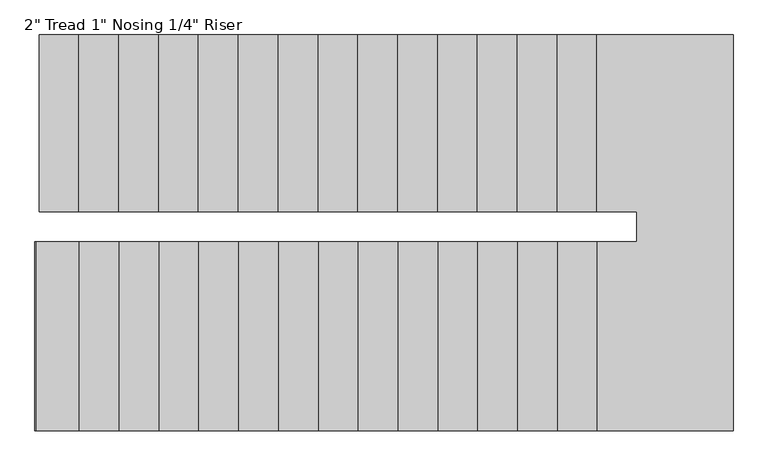
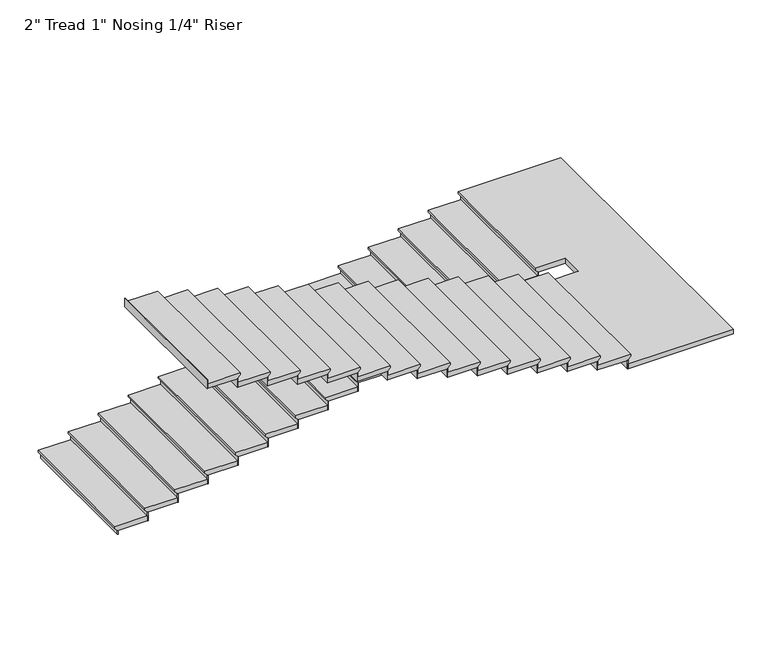
"""IFC4 building model written with IfcOpenShell, lengths in millimetres: stair flight geometry."""

from ifc_helpers import new_model, si_unit, origin, place, context, project, spatial, faceted_brep, source, transform, mapped, element, save


def stair_flight_b8102c9e(model_context):
    return source(origin(), model_context, "Body", "Brep", [
        faceted_brep([(-5254.0891351, 11154.2082924, 6168.39), (-5254.0891351, 11154.2082924, 6187.44), (-5254.0891351, 12506.0715905, 6187.44), (-5254.0891351, 12506.0715905, 6168.39), (-5228.6891351, 11154.2082924, 6142.99), (-5228.6891351, 12506.0715905, 6142.99), (-4923.8891351, 11154.2082924, 6187.44), (-4923.8891351, 12506.0715905, 6187.44), (-5228.6891351, 12506.0715905, 6136.64), (-4923.8891351, 12506.0715905, 6136.64), (-4923.8891351, 11154.2082924, 6136.64), (-5228.6891351, 11154.2082924, 6136.64)], [[[0, 1, 2, 3]], [[4, 0, 3, 5]], [[2, 1, 6, 7]], [[8, 9, 10, 11]], [[2, 7, 9, 8, 5, 3]], [[8, 11, 4, 5]], [[6, 1, 0, 4, 11, 10]], [[7, 6, 10, 9]]]),
        faceted_brep([(-5228.6891351, 11154.2082924, 6136.64), (-5228.6891351, 11154.2082924, 6096.0), (-5222.3391351, 11154.2082924, 6096.0), (-5222.3391351, 11154.2082924, 6136.64), (-5228.6891351, 12506.0715905, 6136.64), (-5222.3391351, 12506.0715905, 6136.64), (-5222.3391351, 12506.0715905, 6096.0), (-5228.6891351, 12506.0715905, 6096.0)], [[[0, 1, 2, 3]], [[4, 5, 6, 7]], [[1, 0, 4, 7]], [[2, 1, 7, 6]], [[3, 2, 6, 5]], [[0, 3, 5, 4]]]),
        faceted_brep([(-4923.8891351, 11154.2082924, 6228.08), (-4923.8891351, 11154.2082924, 6136.64), (-4917.5391351, 11154.2082924, 6136.64), (-4917.5391351, 11154.2082924, 6228.08), (-4923.8891351, 12506.0715905, 6228.08), (-4917.5391351, 12506.0715905, 6228.08), (-4917.5391351, 12506.0715905, 6136.64), (-4923.8891351, 12506.0715905, 6136.64)], [[[0, 1, 2, 3]], [[4, 5, 6, 7]], [[1, 0, 4, 7]], [[2, 1, 7, 6]], [[3, 2, 6, 5]], [[0, 3, 5, 4]]]),
        faceted_brep([(-4949.2891351, 12506.0715905, 6278.88), (-4949.2891351, 11154.2082924, 6278.88), (-4619.0891351, 11154.2082924, 6278.88), (-4619.0891351, 12506.0715905, 6278.88), (-4923.8891351, 12506.0715905, 6228.08), (-4619.0891351, 12506.0715905, 6228.08), (-4619.0891351, 11154.2082924, 6228.08), (-4923.8891351, 11154.2082924, 6228.08), (-4923.8891351, 12506.0715905, 6234.43), (-4949.2891351, 12506.0715905, 6259.83), (-4923.8891351, 11154.2082924, 6234.43), (-4949.2891351, 11154.2082924, 6259.83)], [[[0, 1, 2, 3]], [[4, 5, 6, 7]], [[0, 3, 5, 4, 8, 9]], [[4, 7, 10, 8]], [[2, 1, 11, 10, 7, 6]], [[3, 2, 6, 5]], [[11, 1, 0, 9]], [[10, 11, 9, 8]]]),
        faceted_brep([(-4619.0891351, 11154.2082924, 6319.52), (-4619.0891351, 11154.2082924, 6228.08), (-4612.7391351, 11154.2082924, 6228.08), (-4612.7391351, 11154.2082924, 6319.52), (-4619.0891351, 12506.0715905, 6319.52), (-4612.7391351, 12506.0715905, 6319.52), (-4612.7391351, 12506.0715905, 6228.08), (-4619.0891351, 12506.0715905, 6228.08)], [[[0, 1, 2, 3]], [[4, 5, 6, 7]], [[1, 0, 4, 7]], [[2, 1, 7, 6]], [[3, 2, 6, 5]], [[0, 3, 5, 4]]]),
        faceted_brep([(-4644.4891351, 12506.0715905, 6370.32), (-4644.4891351, 11154.2082924, 6370.32), (-4314.2891351, 11154.2082924, 6370.32), (-4314.2891351, 12506.0715905, 6370.32), (-4619.0891351, 12506.0715905, 6319.52), (-4314.2891351, 12506.0715905, 6319.52), (-4314.2891351, 11154.2082924, 6319.52), (-4619.0891351, 11154.2082924, 6319.52), (-4619.0891351, 12506.0715905, 6325.87), (-4644.4891351, 12506.0715905, 6351.27), (-4619.0891351, 11154.2082924, 6325.87), (-4644.4891351, 11154.2082924, 6351.27)], [[[0, 1, 2, 3]], [[4, 5, 6, 7]], [[0, 3, 5, 4, 8, 9]], [[4, 7, 10, 8]], [[2, 1, 11, 10, 7, 6]], [[3, 2, 6, 5]], [[11, 1, 0, 9]], [[10, 11, 9, 8]]]),
        faceted_brep([(-4314.2891351, 11154.2082924, 6410.96), (-4314.2891351, 11154.2082924, 6319.52), (-4307.9391351, 11154.2082924, 6319.52), (-4307.9391351, 11154.2082924, 6410.96), (-4314.2891351, 12506.0715905, 6410.96), (-4307.9391351, 12506.0715905, 6410.96), (-4307.9391351, 12506.0715905, 6319.52), (-4314.2891351, 12506.0715905, 6319.52)], [[[0, 1, 2, 3]], [[4, 5, 6, 7]], [[1, 0, 4, 7]], [[2, 1, 7, 6]], [[3, 2, 6, 5]], [[0, 3, 5, 4]]]),
        faceted_brep([(-4339.6891351, 12506.0715905, 6461.76), (-4339.6891351, 11154.2082924, 6461.76), (-4009.4891351, 11154.2082924, 6461.76), (-4009.4891351, 12506.0715905, 6461.76), (-4314.2891351, 12506.0715905, 6410.96), (-4009.4891351, 12506.0715905, 6410.96), (-4009.4891351, 11154.2082924, 6410.96), (-4314.2891351, 11154.2082924, 6410.96), (-4314.2891351, 12506.0715905, 6417.31), (-4339.6891351, 12506.0715905, 6442.71), (-4314.2891351, 11154.2082924, 6417.31), (-4339.6891351, 11154.2082924, 6442.71)], [[[0, 1, 2, 3]], [[4, 5, 6, 7]], [[0, 3, 5, 4, 8, 9]], [[4, 7, 10, 8]], [[2, 1, 11, 10, 7, 6]], [[3, 2, 6, 5]], [[11, 1, 0, 9]], [[10, 11, 9, 8]]]),
        faceted_brep([(-4009.4891351, 11154.2082924, 6502.4), (-4009.4891351, 11154.2082924, 6410.96), (-4003.1391351, 11154.2082924, 6410.96), (-4003.1391351, 11154.2082924, 6502.4), (-4009.4891351, 12506.0715905, 6502.4), (-4003.1391351, 12506.0715905, 6502.4), (-4003.1391351, 12506.0715905, 6410.96), (-4009.4891351, 12506.0715905, 6410.96)], [[[0, 1, 2, 3]], [[4, 5, 6, 7]], [[1, 0, 4, 7]], [[2, 1, 7, 6]], [[3, 2, 6, 5]], [[0, 3, 5, 4]]]),
        faceted_brep([(-4034.8891351, 12506.0715905, 6553.2), (-4034.8891351, 11154.2082924, 6553.2), (-3704.6891351, 11154.2082924, 6553.2), (-3704.6891351, 12506.0715905, 6553.2), (-4009.4891351, 12506.0715905, 6502.4), (-3704.6891351, 12506.0715905, 6502.4), (-3704.6891351, 11154.2082924, 6502.4), (-4009.4891351, 11154.2082924, 6502.4), (-4009.4891351, 12506.0715905, 6508.75), (-4034.8891351, 12506.0715905, 6534.15), (-4009.4891351, 11154.2082924, 6508.75), (-4034.8891351, 11154.2082924, 6534.15)], [[[0, 1, 2, 3]], [[4, 5, 6, 7]], [[0, 3, 5, 4, 8, 9]], [[4, 7, 10, 8]], [[2, 1, 11, 10, 7, 6]], [[3, 2, 6, 5]], [[11, 1, 0, 9]], [[10, 11, 9, 8]]]),
        faceted_brep([(-3704.6891351, 11154.2082924, 6593.84), (-3704.6891351, 11154.2082924, 6502.4), (-3698.3391351, 11154.2082924, 6502.4), (-3698.3391351, 11154.2082924, 6593.84), (-3704.6891351, 12506.0715905, 6593.84), (-3698.3391351, 12506.0715905, 6593.84), (-3698.3391351, 12506.0715905, 6502.4), (-3704.6891351, 12506.0715905, 6502.4)], [[[0, 1, 2, 3]], [[4, 5, 6, 7]], [[1, 0, 4, 7]], [[2, 1, 7, 6]], [[3, 2, 6, 5]], [[0, 3, 5, 4]]]),
        faceted_brep([(-3730.0891351, 12506.0715905, 6644.64), (-3730.0891351, 11154.2082924, 6644.64), (-3399.8891351, 11154.2082924, 6644.64), (-3399.8891351, 12506.0715905, 6644.64), (-3704.6891351, 12506.0715905, 6593.84), (-3399.8891351, 12506.0715905, 6593.84), (-3399.8891351, 11154.2082924, 6593.84), (-3704.6891351, 11154.2082924, 6593.84), (-3704.6891351, 12506.0715905, 6600.19), (-3730.0891351, 12506.0715905, 6625.59), (-3704.6891351, 11154.2082924, 6600.19), (-3730.0891351, 11154.2082924, 6625.59)], [[[0, 1, 2, 3]], [[4, 5, 6, 7]], [[0, 3, 5, 4, 8, 9]], [[4, 7, 10, 8]], [[2, 1, 11, 10, 7, 6]], [[3, 2, 6, 5]], [[11, 1, 0, 9]], [[10, 11, 9, 8]]]),
        faceted_brep([(-3399.8891351, 11154.2082924, 6685.28), (-3399.8891351, 11154.2082924, 6593.84), (-3393.5391351, 11154.2082924, 6593.84), (-3393.5391351, 11154.2082924, 6685.28), (-3399.8891351, 12506.0715905, 6685.28), (-3393.5391351, 12506.0715905, 6685.28), (-3393.5391351, 12506.0715905, 6593.84), (-3399.8891351, 12506.0715905, 6593.84)], [[[0, 1, 2, 3]], [[4, 5, 6, 7]], [[1, 0, 4, 7]], [[2, 1, 7, 6]], [[3, 2, 6, 5]], [[0, 3, 5, 4]]]),
        faceted_brep([(-3425.2891351, 12506.0715905, 6736.08), (-3425.2891351, 11154.2082924, 6736.08), (-3095.0891351, 11154.2082924, 6736.08), (-3095.0891351, 12506.0715905, 6736.08), (-3399.8891351, 12506.0715905, 6685.28), (-3095.0891351, 12506.0715905, 6685.28), (-3095.0891351, 11154.2082924, 6685.28), (-3399.8891351, 11154.2082924, 6685.28), (-3399.8891351, 12506.0715905, 6691.63), (-3425.2891351, 12506.0715905, 6717.03), (-3399.8891351, 11154.2082924, 6691.63), (-3425.2891351, 11154.2082924, 6717.03)], [[[0, 1, 2, 3]], [[4, 5, 6, 7]], [[0, 3, 5, 4, 8, 9]], [[4, 7, 10, 8]], [[2, 1, 11, 10, 7, 6]], [[3, 2, 6, 5]], [[11, 1, 0, 9]], [[10, 11, 9, 8]]]),
        faceted_brep([(-3095.0891351, 11154.2082924, 6776.72), (-3095.0891351, 11154.2082924, 6685.28), (-3088.7391351, 11154.2082924, 6685.28), (-3088.7391351, 11154.2082924, 6776.72), (-3095.0891351, 12506.0715905, 6776.72), (-3088.7391351, 12506.0715905, 6776.72), (-3088.7391351, 12506.0715905, 6685.28), (-3095.0891351, 12506.0715905, 6685.28)], [[[0, 1, 2, 3]], [[4, 5, 6, 7]], [[1, 0, 4, 7]], [[2, 1, 7, 6]], [[3, 2, 6, 5]], [[0, 3, 5, 4]]]),
        faceted_brep([(-3120.4891351, 12506.0715905, 6827.52), (-3120.4891351, 11154.2082924, 6827.52), (-2790.2891351, 11154.2082924, 6827.52), (-2790.2891351, 12506.0715905, 6827.52), (-3095.0891351, 12506.0715905, 6776.72), (-2790.2891351, 12506.0715905, 6776.72), (-2790.2891351, 11154.2082924, 6776.72), (-3095.0891351, 11154.2082924, 6776.72), (-3095.0891351, 12506.0715905, 6783.07), (-3120.4891351, 12506.0715905, 6808.47), (-3095.0891351, 11154.2082924, 6783.07), (-3120.4891351, 11154.2082924, 6808.47)], [[[0, 1, 2, 3]], [[4, 5, 6, 7]], [[0, 3, 5, 4, 8, 9]], [[4, 7, 10, 8]], [[2, 1, 11, 10, 7, 6]], [[3, 2, 6, 5]], [[11, 1, 0, 9]], [[10, 11, 9, 8]]]),
        faceted_brep([(-2790.2891351, 11154.2082924, 6868.16), (-2790.2891351, 11154.2082924, 6776.72), (-2783.9391351, 11154.2082924, 6776.72), (-2783.9391351, 11154.2082924, 6868.16), (-2790.2891351, 12506.0715905, 6868.16), (-2783.9391351, 12506.0715905, 6868.16), (-2783.9391351, 12506.0715905, 6776.72), (-2790.2891351, 12506.0715905, 6776.72)], [[[0, 1, 2, 3]], [[4, 5, 6, 7]], [[1, 0, 4, 7]], [[2, 1, 7, 6]], [[3, 2, 6, 5]], [[0, 3, 5, 4]]]),
        faceted_brep([(-2815.6891351, 12506.0715905, 6918.96), (-2815.6891351, 11154.2082924, 6918.96), (-2485.4891351, 11154.2082924, 6918.96), (-2485.4891351, 12506.0715905, 6918.96), (-2790.2891351, 12506.0715905, 6868.16), (-2485.4891351, 12506.0715905, 6868.16), (-2485.4891351, 11154.2082924, 6868.16), (-2790.2891351, 11154.2082924, 6868.16), (-2790.2891351, 12506.0715905, 6874.51), (-2815.6891351, 12506.0715905, 6899.91), (-2790.2891351, 11154.2082924, 6874.51), (-2815.6891351, 11154.2082924, 6899.91)], [[[0, 1, 2, 3]], [[4, 5, 6, 7]], [[0, 3, 5, 4, 8, 9]], [[4, 7, 10, 8]], [[2, 1, 11, 10, 7, 6]], [[3, 2, 6, 5]], [[11, 1, 0, 9]], [[10, 11, 9, 8]]]),
        faceted_brep([(-2485.4891351, 11154.2082924, 6959.6), (-2485.4891351, 11154.2082924, 6868.16), (-2479.1391351, 11154.2082924, 6868.16), (-2479.1391351, 11154.2082924, 6959.6), (-2485.4891351, 12506.0715905, 6959.6), (-2479.1391351, 12506.0715905, 6959.6), (-2479.1391351, 12506.0715905, 6868.16), (-2485.4891351, 12506.0715905, 6868.16)], [[[0, 1, 2, 3]], [[4, 5, 6, 7]], [[1, 0, 4, 7]], [[2, 1, 7, 6]], [[3, 2, 6, 5]], [[0, 3, 5, 4]]]),
        faceted_brep([(-2510.8891351, 12506.0715905, 7010.4), (-2510.8891351, 11154.2082924, 7010.4), (-2180.6891351, 11154.2082924, 7010.4), (-2180.6891351, 12506.0715905, 7010.4), (-2485.4891351, 12506.0715905, 6959.6), (-2180.6891351, 12506.0715905, 6959.6), (-2180.6891351, 11154.2082924, 6959.6), (-2485.4891351, 11154.2082924, 6959.6), (-2485.4891351, 12506.0715905, 6965.95), (-2510.8891351, 12506.0715905, 6991.35), (-2485.4891351, 11154.2082924, 6965.95), (-2510.8891351, 11154.2082924, 6991.35)], [[[0, 1, 2, 3]], [[4, 5, 6, 7]], [[0, 3, 5, 4, 8, 9]], [[4, 7, 10, 8]], [[2, 1, 11, 10, 7, 6]], [[3, 2, 6, 5]], [[11, 1, 0, 9]], [[10, 11, 9, 8]]]),
        faceted_brep([(-2180.6891351, 11154.2082924, 7051.04), (-2180.6891351, 11154.2082924, 6959.6), (-2174.3391351, 11154.2082924, 6959.6), (-2174.3391351, 11154.2082924, 7051.04), (-2180.6891351, 12506.0715905, 7051.04), (-2174.3391351, 12506.0715905, 7051.04), (-2174.3391351, 12506.0715905, 6959.6), (-2180.6891351, 12506.0715905, 6959.6)], [[[0, 1, 2, 3]], [[4, 5, 6, 7]], [[1, 0, 4, 7]], [[2, 1, 7, 6]], [[3, 2, 6, 5]], [[0, 3, 5, 4]]]),
        faceted_brep([(-2206.0891351, 12506.0715905, 7101.84), (-2206.0891351, 11154.2082924, 7101.84), (-1875.8891351, 11154.2082924, 7101.84), (-1875.8891351, 12506.0715905, 7101.84), (-2180.6891351, 12506.0715905, 7051.04), (-1875.8891351, 12506.0715905, 7051.04), (-1875.8891351, 11154.2082924, 7051.04), (-2180.6891351, 11154.2082924, 7051.04), (-2180.6891351, 12506.0715905, 7057.39), (-2206.0891351, 12506.0715905, 7082.79), (-2180.6891351, 11154.2082924, 7057.39), (-2206.0891351, 11154.2082924, 7082.79)], [[[0, 1, 2, 3]], [[4, 5, 6, 7]], [[0, 3, 5, 4, 8, 9]], [[4, 7, 10, 8]], [[2, 1, 11, 10, 7, 6]], [[3, 2, 6, 5]], [[11, 1, 0, 9]], [[10, 11, 9, 8]]]),
        faceted_brep([(-1875.8891351, 11154.2082924, 7142.48), (-1875.8891351, 11154.2082924, 7051.04), (-1869.5391351, 11154.2082924, 7051.04), (-1869.5391351, 11154.2082924, 7142.48), (-1875.8891351, 12506.0715905, 7142.48), (-1869.5391351, 12506.0715905, 7142.48), (-1869.5391351, 12506.0715905, 7051.04), (-1875.8891351, 12506.0715905, 7051.04)], [[[0, 1, 2, 3]], [[4, 5, 6, 7]], [[1, 0, 4, 7]], [[2, 1, 7, 6]], [[3, 2, 6, 5]], [[0, 3, 5, 4]]]),
        faceted_brep([(-1901.2891351, 12506.0715905, 7193.28), (-1901.2891351, 11154.2082924, 7193.28), (-1571.0891351, 11154.2082924, 7193.28), (-1571.0891351, 12506.0715905, 7193.28), (-1875.8891351, 12506.0715905, 7142.48), (-1571.0891351, 12506.0715905, 7142.48), (-1571.0891351, 11154.2082924, 7142.48), (-1875.8891351, 11154.2082924, 7142.48), (-1875.8891351, 12506.0715905, 7148.83), (-1901.2891351, 12506.0715905, 7174.23), (-1875.8891351, 11154.2082924, 7148.83), (-1901.2891351, 11154.2082924, 7174.23)], [[[0, 1, 2, 3]], [[4, 5, 6, 7]], [[0, 3, 5, 4, 8, 9]], [[4, 7, 10, 8]], [[2, 1, 11, 10, 7, 6]], [[3, 2, 6, 5]], [[11, 1, 0, 9]], [[10, 11, 9, 8]]]),
        faceted_brep([(-1571.0891351, 11154.2082924, 7233.92), (-1571.0891351, 11154.2082924, 7142.48), (-1564.7391351, 11154.2082924, 7142.48), (-1564.7391351, 11154.2082924, 7233.92), (-1571.0891351, 12506.0715905, 7233.92), (-1564.7391351, 12506.0715905, 7233.92), (-1564.7391351, 12506.0715905, 7142.48), (-1571.0891351, 12506.0715905, 7142.48)], [[[0, 1, 2, 3]], [[4, 5, 6, 7]], [[1, 0, 4, 7]], [[2, 1, 7, 6]], [[3, 2, 6, 5]], [[0, 3, 5, 4]]]),
        faceted_brep([(-1596.4891351, 12506.0715905, 7284.72), (-1596.4891351, 11154.2082924, 7284.72), (-1266.2891351, 11154.2082924, 7284.72), (-1266.2891351, 12506.0715905, 7284.72), (-1571.0891351, 12506.0715905, 7233.92), (-1266.2891351, 12506.0715905, 7233.92), (-1266.2891351, 11154.2082924, 7233.92), (-1571.0891351, 11154.2082924, 7233.92), (-1571.0891351, 12506.0715905, 7240.27), (-1596.4891351, 12506.0715905, 7265.67), (-1571.0891351, 11154.2082924, 7240.27), (-1596.4891351, 11154.2082924, 7265.67)], [[[0, 1, 2, 3]], [[4, 5, 6, 7]], [[0, 3, 5, 4, 8, 9]], [[4, 7, 10, 8]], [[2, 1, 11, 10, 7, 6]], [[3, 2, 6, 5]], [[11, 1, 0, 9]], [[10, 11, 9, 8]]]),
        faceted_brep([(-1266.2891351, 11154.2082924, 7325.36), (-1266.2891351, 11154.2082924, 7233.92), (-1259.9391351, 11154.2082924, 7233.92), (-1259.9391351, 11154.2082924, 7325.36), (-1266.2891351, 12506.0715905, 7325.36), (-1259.9391351, 12506.0715905, 7325.36), (-1259.9391351, 12506.0715905, 7233.92), (-1266.2891351, 12506.0715905, 7233.92)], [[[0, 1, 2, 3]], [[4, 5, 6, 7]], [[1, 0, 4, 7]], [[2, 1, 7, 6]], [[3, 2, 6, 5]], [[0, 3, 5, 4]]]),
        faceted_brep([(-1291.6891351, 12506.0715905, 7376.16), (-1291.6891351, 11154.2082924, 7376.16), (-961.4891351, 11154.2082924, 7376.16), (-961.4891351, 12506.0715905, 7376.16), (-1266.2891351, 12506.0715905, 7325.36), (-961.4891351, 12506.0715905, 7325.36), (-961.4891351, 11154.2082924, 7325.36), (-1266.2891351, 11154.2082924, 7325.36), (-1266.2891351, 12506.0715905, 7331.71), (-1291.6891351, 12506.0715905, 7357.11), (-1266.2891351, 11154.2082924, 7331.71), (-1291.6891351, 11154.2082924, 7357.11)], [[[0, 1, 2, 3]], [[4, 5, 6, 7]], [[0, 3, 5, 4, 8, 9]], [[4, 7, 10, 8]], [[2, 1, 11, 10, 7, 6]], [[3, 2, 6, 5]], [[11, 1, 0, 9]], [[10, 11, 9, 8]]]),
        faceted_brep([(-961.4891351, 11154.2082924, 7416.8), (-961.4891351, 11154.2082924, 7325.36), (-955.1391351, 11154.2082924, 7325.36), (-955.1391351, 11154.2082924, 7416.8), (-961.4891351, 12506.0715905, 7416.8), (-955.1391351, 12506.0715905, 7416.8), (-955.1391351, 12506.0715905, 7325.36), (-961.4891351, 12506.0715905, 7325.36)], [[[0, 1, 2, 3]], [[4, 5, 6, 7]], [[1, 0, 4, 7]], [[2, 1, 7, 6]], [[3, 2, 6, 5]], [[0, 3, 5, 4]]]),
        faceted_brep([(-1012.2891351, 9478.4949943, 7467.6), (54.5108649, 9478.4949943, 7467.6), (54.5108649, 12506.0715905, 7467.6), (-986.8891351, 12506.0715905, 7467.6), (-986.8891351, 11154.2082924, 7467.6), (-682.0891351, 11154.2082924, 7467.6), (-682.0891351, 10925.6082924, 7467.6), (-1012.2891351, 10925.6082924, 7467.6), (54.5108649, 9478.4949943, 7416.8), (-1012.2891351, 9478.4949943, 7416.8), (-1012.2891351, 10925.6082924, 7416.8), (-682.0891351, 10925.6082924, 7416.8), (-682.0891351, 11154.2082924, 7416.8), (-961.4891351, 11154.2082924, 7416.8), (-961.4891351, 12506.0715905, 7416.8), (54.5108649, 12506.0715905, 7416.8), (-961.4891351, 12506.0715905, 7423.15), (-986.8891351, 12506.0715905, 7448.55), (-961.4891351, 11154.2082924, 7423.15), (-986.8891351, 11154.2082924, 7448.55)], [[[0, 1, 2, 3, 4, 5, 6, 7]], [[8, 9, 10, 11, 12, 13, 14, 15]], [[1, 0, 9, 8]], [[2, 1, 8, 15]], [[3, 2, 15, 14, 16, 17]], [[14, 13, 18, 16]], [[5, 4, 19, 18, 13, 12]], [[6, 5, 12, 11]], [[7, 6, 11, 10]], [[0, 7, 10, 9]], [[19, 4, 3, 17]], [[18, 19, 17, 16]]]),
        faceted_brep([(-1012.2891351, 10925.6082924, 7508.24), (-1012.2891351, 10925.6082924, 7416.8), (-1018.6391351, 10925.6082924, 7416.8), (-1018.6391351, 10925.6082924, 7508.24), (-1012.2891351, 9478.4949943, 7508.24), (-1018.6391351, 9478.4949943, 7508.24), (-1018.6391351, 9478.4949943, 7416.8), (-1012.2891351, 9478.4949943, 7416.8)], [[[0, 1, 2, 3]], [[4, 5, 6, 7]], [[1, 0, 4, 7]], [[2, 1, 7, 6]], [[3, 2, 6, 5]], [[0, 3, 5, 4]]]),
        faceted_brep([(-986.8891351, 9478.4949943, 7559.04), (-986.8891351, 10925.6082924, 7559.04), (-1317.0891351, 10925.6082924, 7559.04), (-1317.0891351, 9478.4949943, 7559.04), (-1012.2891351, 9478.4949943, 7508.24), (-1317.0891351, 9478.4949943, 7508.24), (-1317.0891351, 10925.6082924, 7508.24), (-1012.2891351, 10925.6082924, 7508.24), (-1012.2891351, 9478.4949943, 7514.59), (-986.8891351, 9478.4949943, 7539.99), (-1012.2891351, 10925.6082924, 7514.59), (-986.8891351, 10925.6082924, 7539.99)], [[[0, 1, 2, 3]], [[4, 5, 6, 7]], [[0, 3, 5, 4, 8, 9]], [[4, 7, 10, 8]], [[2, 1, 11, 10, 7, 6]], [[3, 2, 6, 5]], [[11, 1, 0, 9]], [[10, 11, 9, 8]]]),
        faceted_brep([(-1317.0891351, 10925.6082924, 7599.68), (-1317.0891351, 10925.6082924, 7508.24), (-1323.4391351, 10925.6082924, 7508.24), (-1323.4391351, 10925.6082924, 7599.68), (-1317.0891351, 9478.4949943, 7599.68), (-1323.4391351, 9478.4949943, 7599.68), (-1323.4391351, 9478.4949943, 7508.24), (-1317.0891351, 9478.4949943, 7508.24)], [[[0, 1, 2, 3]], [[4, 5, 6, 7]], [[1, 0, 4, 7]], [[2, 1, 7, 6]], [[3, 2, 6, 5]], [[0, 3, 5, 4]]]),
        faceted_brep([(-1291.6891351, 9478.4949943, 7650.48), (-1291.6891351, 10925.6082924, 7650.48), (-1621.8891351, 10925.6082924, 7650.48), (-1621.8891351, 9478.4949943, 7650.48), (-1317.0891351, 9478.4949943, 7599.68), (-1621.8891351, 9478.4949943, 7599.68), (-1621.8891351, 10925.6082924, 7599.68), (-1317.0891351, 10925.6082924, 7599.68), (-1317.0891351, 9478.4949943, 7606.03), (-1291.6891351, 9478.4949943, 7631.43), (-1317.0891351, 10925.6082924, 7606.03), (-1291.6891351, 10925.6082924, 7631.43)], [[[0, 1, 2, 3]], [[4, 5, 6, 7]], [[0, 3, 5, 4, 8, 9]], [[4, 7, 10, 8]], [[2, 1, 11, 10, 7, 6]], [[3, 2, 6, 5]], [[11, 1, 0, 9]], [[10, 11, 9, 8]]]),
        faceted_brep([(-1621.8891351, 10925.6082924, 7691.12), (-1621.8891351, 10925.6082924, 7599.68), (-1628.2391351, 10925.6082924, 7599.68), (-1628.2391351, 10925.6082924, 7691.12), (-1621.8891351, 9478.4949943, 7691.12), (-1628.2391351, 9478.4949943, 7691.12), (-1628.2391351, 9478.4949943, 7599.68), (-1621.8891351, 9478.4949943, 7599.68)], [[[0, 1, 2, 3]], [[4, 5, 6, 7]], [[1, 0, 4, 7]], [[2, 1, 7, 6]], [[3, 2, 6, 5]], [[0, 3, 5, 4]]]),
        faceted_brep([(-1596.4891351, 9478.4949943, 7741.92), (-1596.4891351, 10925.6082924, 7741.92), (-1926.6891351, 10925.6082924, 7741.92), (-1926.6891351, 9478.4949943, 7741.92), (-1621.8891351, 9478.4949943, 7691.12), (-1926.6891351, 9478.4949943, 7691.12), (-1926.6891351, 10925.6082924, 7691.12), (-1621.8891351, 10925.6082924, 7691.12), (-1621.8891351, 9478.4949943, 7697.47), (-1596.4891351, 9478.4949943, 7722.87), (-1621.8891351, 10925.6082924, 7697.47), (-1596.4891351, 10925.6082924, 7722.87)], [[[0, 1, 2, 3]], [[4, 5, 6, 7]], [[0, 3, 5, 4, 8, 9]], [[4, 7, 10, 8]], [[2, 1, 11, 10, 7, 6]], [[3, 2, 6, 5]], [[11, 1, 0, 9]], [[10, 11, 9, 8]]]),
        faceted_brep([(-1926.6891351, 10925.6082924, 7782.56), (-1926.6891351, 10925.6082924, 7691.12), (-1933.0391351, 10925.6082924, 7691.12), (-1933.0391351, 10925.6082924, 7782.56), (-1926.6891351, 9478.4949943, 7782.56), (-1933.0391351, 9478.4949943, 7782.56), (-1933.0391351, 9478.4949943, 7691.12), (-1926.6891351, 9478.4949943, 7691.12)], [[[0, 1, 2, 3]], [[4, 5, 6, 7]], [[1, 0, 4, 7]], [[2, 1, 7, 6]], [[3, 2, 6, 5]], [[0, 3, 5, 4]]]),
        faceted_brep([(-1901.2891351, 9478.4949943, 7833.36), (-1901.2891351, 10925.6082924, 7833.36), (-2231.4891351, 10925.6082924, 7833.36), (-2231.4891351, 9478.4949943, 7833.36), (-1926.6891351, 9478.4949943, 7782.56), (-2231.4891351, 9478.4949943, 7782.56), (-2231.4891351, 10925.6082924, 7782.56), (-1926.6891351, 10925.6082924, 7782.56), (-1926.6891351, 9478.4949943, 7788.91), (-1901.2891351, 9478.4949943, 7814.31), (-1926.6891351, 10925.6082924, 7788.91), (-1901.2891351, 10925.6082924, 7814.31)], [[[0, 1, 2, 3]], [[4, 5, 6, 7]], [[0, 3, 5, 4, 8, 9]], [[4, 7, 10, 8]], [[2, 1, 11, 10, 7, 6]], [[3, 2, 6, 5]], [[11, 1, 0, 9]], [[10, 11, 9, 8]]]),
        faceted_brep([(-2231.4891351, 10925.6082924, 7874.0), (-2231.4891351, 10925.6082924, 7782.56), (-2237.8391351, 10925.6082924, 7782.56), (-2237.8391351, 10925.6082924, 7874.0), (-2231.4891351, 9478.4949943, 7874.0), (-2237.8391351, 9478.4949943, 7874.0), (-2237.8391351, 9478.4949943, 7782.56), (-2231.4891351, 9478.4949943, 7782.56)], [[[0, 1, 2, 3]], [[4, 5, 6, 7]], [[1, 0, 4, 7]], [[2, 1, 7, 6]], [[3, 2, 6, 5]], [[0, 3, 5, 4]]]),
        faceted_brep([(-2206.0891351, 9478.4949943, 7924.8), (-2206.0891351, 10925.6082924, 7924.8), (-2536.2891351, 10925.6082924, 7924.8), (-2536.2891351, 9478.4949943, 7924.8), (-2231.4891351, 9478.4949943, 7874.0), (-2536.2891351, 9478.4949943, 7874.0), (-2536.2891351, 10925.6082924, 7874.0), (-2231.4891351, 10925.6082924, 7874.0), (-2231.4891351, 9478.4949943, 7880.35), (-2206.0891351, 9478.4949943, 7905.75), (-2231.4891351, 10925.6082924, 7880.35), (-2206.0891351, 10925.6082924, 7905.75)], [[[0, 1, 2, 3]], [[4, 5, 6, 7]], [[0, 3, 5, 4, 8, 9]], [[4, 7, 10, 8]], [[2, 1, 11, 10, 7, 6]], [[3, 2, 6, 5]], [[11, 1, 0, 9]], [[10, 11, 9, 8]]]),
        faceted_brep([(-2536.2891351, 10925.6082924, 7965.44), (-2536.2891351, 10925.6082924, 7874.0), (-2542.6391351, 10925.6082924, 7874.0), (-2542.6391351, 10925.6082924, 7965.44), (-2536.2891351, 9478.4949943, 7965.44), (-2542.6391351, 9478.4949943, 7965.44), (-2542.6391351, 9478.4949943, 7874.0), (-2536.2891351, 9478.4949943, 7874.0)], [[[0, 1, 2, 3]], [[4, 5, 6, 7]], [[1, 0, 4, 7]], [[2, 1, 7, 6]], [[3, 2, 6, 5]], [[0, 3, 5, 4]]]),
        faceted_brep([(-2510.8891351, 9478.4949943, 8016.24), (-2510.8891351, 10925.6082924, 8016.24), (-2841.0891351, 10925.6082924, 8016.24), (-2841.0891351, 9478.4949943, 8016.24), (-2536.2891351, 9478.4949943, 7965.44), (-2841.0891351, 9478.4949943, 7965.44), (-2841.0891351, 10925.6082924, 7965.44), (-2536.2891351, 10925.6082924, 7965.44), (-2536.2891351, 9478.4949943, 7971.79), (-2510.8891351, 9478.4949943, 7997.19), (-2536.2891351, 10925.6082924, 7971.79), (-2510.8891351, 10925.6082924, 7997.19)], [[[0, 1, 2, 3]], [[4, 5, 6, 7]], [[0, 3, 5, 4, 8, 9]], [[4, 7, 10, 8]], [[2, 1, 11, 10, 7, 6]], [[3, 2, 6, 5]], [[11, 1, 0, 9]], [[10, 11, 9, 8]]]),
        faceted_brep([(-2841.0891351, 10925.6082924, 8056.88), (-2841.0891351, 10925.6082924, 7965.44), (-2847.4391351, 10925.6082924, 7965.44), (-2847.4391351, 10925.6082924, 8056.88), (-2841.0891351, 9478.4949943, 8056.88), (-2847.4391351, 9478.4949943, 8056.88), (-2847.4391351, 9478.4949943, 7965.44), (-2841.0891351, 9478.4949943, 7965.44)], [[[0, 1, 2, 3]], [[4, 5, 6, 7]], [[1, 0, 4, 7]], [[2, 1, 7, 6]], [[3, 2, 6, 5]], [[0, 3, 5, 4]]]),
        faceted_brep([(-2815.6891351, 9478.4949943, 8107.68), (-2815.6891351, 10925.6082924, 8107.68), (-3145.8891351, 10925.6082924, 8107.68), (-3145.8891351, 9478.4949943, 8107.68), (-2841.0891351, 9478.4949943, 8056.88), (-3145.8891351, 9478.4949943, 8056.88), (-3145.8891351, 10925.6082924, 8056.88), (-2841.0891351, 10925.6082924, 8056.88), (-2841.0891351, 9478.4949943, 8063.23), (-2815.6891351, 9478.4949943, 8088.63), (-2841.0891351, 10925.6082924, 8063.23), (-2815.6891351, 10925.6082924, 8088.63)], [[[0, 1, 2, 3]], [[4, 5, 6, 7]], [[0, 3, 5, 4, 8, 9]], [[4, 7, 10, 8]], [[2, 1, 11, 10, 7, 6]], [[3, 2, 6, 5]], [[11, 1, 0, 9]], [[10, 11, 9, 8]]]),
        faceted_brep([(-3145.8891351, 10925.6082924, 8148.32), (-3145.8891351, 10925.6082924, 8056.88), (-3152.2391351, 10925.6082924, 8056.88), (-3152.2391351, 10925.6082924, 8148.32), (-3145.8891351, 9478.4949943, 8148.32), (-3152.2391351, 9478.4949943, 8148.32), (-3152.2391351, 9478.4949943, 8056.88), (-3145.8891351, 9478.4949943, 8056.88)], [[[0, 1, 2, 3]], [[4, 5, 6, 7]], [[1, 0, 4, 7]], [[2, 1, 7, 6]], [[3, 2, 6, 5]], [[0, 3, 5, 4]]]),
        faceted_brep([(-3120.4891351, 9478.4949943, 8199.12), (-3120.4891351, 10925.6082924, 8199.12), (-3450.6891351, 10925.6082924, 8199.12), (-3450.6891351, 9478.4949943, 8199.12), (-3145.8891351, 9478.4949943, 8148.32), (-3450.6891351, 9478.4949943, 8148.32), (-3450.6891351, 10925.6082924, 8148.32), (-3145.8891351, 10925.6082924, 8148.32), (-3145.8891351, 9478.4949943, 8154.67), (-3120.4891351, 9478.4949943, 8180.07), (-3145.8891351, 10925.6082924, 8154.67), (-3120.4891351, 10925.6082924, 8180.07)], [[[0, 1, 2, 3]], [[4, 5, 6, 7]], [[0, 3, 5, 4, 8, 9]], [[4, 7, 10, 8]], [[2, 1, 11, 10, 7, 6]], [[3, 2, 6, 5]], [[11, 1, 0, 9]], [[10, 11, 9, 8]]]),
        faceted_brep([(-3450.6891351, 10925.6082924, 8239.76), (-3450.6891351, 10925.6082924, 8148.32), (-3457.0391351, 10925.6082924, 8148.32), (-3457.0391351, 10925.6082924, 8239.76), (-3450.6891351, 9478.4949943, 8239.76), (-3457.0391351, 9478.4949943, 8239.76), (-3457.0391351, 9478.4949943, 8148.32), (-3450.6891351, 9478.4949943, 8148.32)], [[[0, 1, 2, 3]], [[4, 5, 6, 7]], [[1, 0, 4, 7]], [[2, 1, 7, 6]], [[3, 2, 6, 5]], [[0, 3, 5, 4]]]),
        faceted_brep([(-3425.2891351, 9478.4949943, 8290.56), (-3425.2891351, 10925.6082924, 8290.56), (-3755.4891351, 10925.6082924, 8290.56), (-3755.4891351, 9478.4949943, 8290.56), (-3450.6891351, 9478.4949943, 8239.76), (-3755.4891351, 9478.4949943, 8239.76), (-3755.4891351, 10925.6082924, 8239.76), (-3450.6891351, 10925.6082924, 8239.76), (-3450.6891351, 9478.4949943, 8246.11), (-3425.2891351, 9478.4949943, 8271.51), (-3450.6891351, 10925.6082924, 8246.11), (-3425.2891351, 10925.6082924, 8271.51)], [[[0, 1, 2, 3]], [[4, 5, 6, 7]], [[0, 3, 5, 4, 8, 9]], [[4, 7, 10, 8]], [[2, 1, 11, 10, 7, 6]], [[3, 2, 6, 5]], [[11, 1, 0, 9]], [[10, 11, 9, 8]]]),
        faceted_brep([(-3755.4891351, 10925.6082924, 8331.2), (-3755.4891351, 10925.6082924, 8239.76), (-3761.8391351, 10925.6082924, 8239.76), (-3761.8391351, 10925.6082924, 8331.2), (-3755.4891351, 9478.4949943, 8331.2), (-3761.8391351, 9478.4949943, 8331.2), (-3761.8391351, 9478.4949943, 8239.76), (-3755.4891351, 9478.4949943, 8239.76)], [[[0, 1, 2, 3]], [[4, 5, 6, 7]], [[1, 0, 4, 7]], [[2, 1, 7, 6]], [[3, 2, 6, 5]], [[0, 3, 5, 4]]]),
        faceted_brep([(-3730.0891351, 9478.4949943, 8382.0), (-3730.0891351, 10925.6082924, 8382.0), (-4060.2891351, 10925.6082924, 8382.0), (-4060.2891351, 9478.4949943, 8382.0), (-3755.4891351, 9478.4949943, 8331.2), (-4060.2891351, 9478.4949943, 8331.2), (-4060.2891351, 10925.6082924, 8331.2), (-3755.4891351, 10925.6082924, 8331.2), (-3755.4891351, 9478.4949943, 8337.55), (-3730.0891351, 9478.4949943, 8362.95), (-3755.4891351, 10925.6082924, 8337.55), (-3730.0891351, 10925.6082924, 8362.95)], [[[0, 1, 2, 3]], [[4, 5, 6, 7]], [[0, 3, 5, 4, 8, 9]], [[4, 7, 10, 8]], [[2, 1, 11, 10, 7, 6]], [[3, 2, 6, 5]], [[11, 1, 0, 9]], [[10, 11, 9, 8]]]),
        faceted_brep([(-4060.2891351, 10925.6082924, 8422.64), (-4060.2891351, 10925.6082924, 8331.2), (-4066.6391351, 10925.6082924, 8331.2), (-4066.6391351, 10925.6082924, 8422.64), (-4060.2891351, 9478.4949943, 8422.64), (-4066.6391351, 9478.4949943, 8422.64), (-4066.6391351, 9478.4949943, 8331.2), (-4060.2891351, 9478.4949943, 8331.2)], [[[0, 1, 2, 3]], [[4, 5, 6, 7]], [[1, 0, 4, 7]], [[2, 1, 7, 6]], [[3, 2, 6, 5]], [[0, 3, 5, 4]]]),
        faceted_brep([(-4034.8891351, 9478.4949943, 8473.44), (-4034.8891351, 10925.6082924, 8473.44), (-4365.0891351, 10925.6082924, 8473.44), (-4365.0891351, 9478.4949943, 8473.44), (-4060.2891351, 9478.4949943, 8422.64), (-4365.0891351, 9478.4949943, 8422.64), (-4365.0891351, 10925.6082924, 8422.64), (-4060.2891351, 10925.6082924, 8422.64), (-4060.2891351, 9478.4949943, 8428.99), (-4034.8891351, 9478.4949943, 8454.39), (-4060.2891351, 10925.6082924, 8428.99), (-4034.8891351, 10925.6082924, 8454.39)], [[[0, 1, 2, 3]], [[4, 5, 6, 7]], [[0, 3, 5, 4, 8, 9]], [[4, 7, 10, 8]], [[2, 1, 11, 10, 7, 6]], [[3, 2, 6, 5]], [[11, 1, 0, 9]], [[10, 11, 9, 8]]]),
        faceted_brep([(-4365.0891351, 10925.6082924, 8514.08), (-4365.0891351, 10925.6082924, 8422.64), (-4371.4391351, 10925.6082924, 8422.64), (-4371.4391351, 10925.6082924, 8514.08), (-4365.0891351, 9478.4949943, 8514.08), (-4371.4391351, 9478.4949943, 8514.08), (-4371.4391351, 9478.4949943, 8422.64), (-4365.0891351, 9478.4949943, 8422.64)], [[[0, 1, 2, 3]], [[4, 5, 6, 7]], [[1, 0, 4, 7]], [[2, 1, 7, 6]], [[3, 2, 6, 5]], [[0, 3, 5, 4]]]),
        faceted_brep([(-4339.6891351, 9478.4949943, 8564.88), (-4339.6891351, 10925.6082924, 8564.88), (-4669.8891351, 10925.6082924, 8564.88), (-4669.8891351, 9478.4949943, 8564.88), (-4365.0891351, 9478.4949943, 8514.08), (-4669.8891351, 9478.4949943, 8514.08), (-4669.8891351, 10925.6082924, 8514.08), (-4365.0891351, 10925.6082924, 8514.08), (-4365.0891351, 9478.4949943, 8520.43), (-4339.6891351, 9478.4949943, 8545.83), (-4365.0891351, 10925.6082924, 8520.43), (-4339.6891351, 10925.6082924, 8545.83)], [[[0, 1, 2, 3]], [[4, 5, 6, 7]], [[0, 3, 5, 4, 8, 9]], [[4, 7, 10, 8]], [[2, 1, 11, 10, 7, 6]], [[3, 2, 6, 5]], [[11, 1, 0, 9]], [[10, 11, 9, 8]]]),
        faceted_brep([(-4669.8891351, 10925.6082924, 8605.52), (-4669.8891351, 10925.6082924, 8514.08), (-4676.2391351, 10925.6082924, 8514.08), (-4676.2391351, 10925.6082924, 8605.52), (-4669.8891351, 9478.4949943, 8605.52), (-4676.2391351, 9478.4949943, 8605.52), (-4676.2391351, 9478.4949943, 8514.08), (-4669.8891351, 9478.4949943, 8514.08)], [[[0, 1, 2, 3]], [[4, 5, 6, 7]], [[1, 0, 4, 7]], [[2, 1, 7, 6]], [[3, 2, 6, 5]], [[0, 3, 5, 4]]]),
        faceted_brep([(-4644.4891351, 9478.4949943, 8656.32), (-4644.4891351, 10925.6082924, 8656.32), (-4974.6891351, 10925.6082924, 8656.32), (-4974.6891351, 9478.4949943, 8656.32), (-4669.8891351, 9478.4949943, 8605.52), (-4974.6891351, 9478.4949943, 8605.52), (-4974.6891351, 10925.6082924, 8605.52), (-4669.8891351, 10925.6082924, 8605.52), (-4669.8891351, 9478.4949943, 8611.87), (-4644.4891351, 9478.4949943, 8637.27), (-4669.8891351, 10925.6082924, 8611.87), (-4644.4891351, 10925.6082924, 8637.27)], [[[0, 1, 2, 3]], [[4, 5, 6, 7]], [[0, 3, 5, 4, 8, 9]], [[4, 7, 10, 8]], [[2, 1, 11, 10, 7, 6]], [[3, 2, 6, 5]], [[11, 1, 0, 9]], [[10, 11, 9, 8]]]),
        faceted_brep([(-4974.6891351, 10925.6082924, 8696.96), (-4974.6891351, 10925.6082924, 8605.52), (-4981.0391351, 10925.6082924, 8605.52), (-4981.0391351, 10925.6082924, 8696.96), (-4974.6891351, 9478.4949943, 8696.96), (-4981.0391351, 9478.4949943, 8696.96), (-4981.0391351, 9478.4949943, 8605.52), (-4974.6891351, 9478.4949943, 8605.52)], [[[0, 1, 2, 3]], [[4, 5, 6, 7]], [[1, 0, 4, 7]], [[2, 1, 7, 6]], [[3, 2, 6, 5]], [[0, 3, 5, 4]]]),
        faceted_brep([(-5279.4891351, 10925.6082924, 8788.4), (-5279.4891351, 10925.6082924, 8696.96), (-5285.8391351, 10925.6082924, 8696.96), (-5285.8391351, 10925.6082924, 8788.4), (-5279.4891351, 9478.4949943, 8788.4), (-5285.8391351, 9478.4949943, 8788.4), (-5285.8391351, 9478.4949943, 8696.96), (-5279.4891351, 9478.4949943, 8696.96)], [[[0, 1, 2, 3]], [[4, 5, 6, 7]], [[1, 0, 4, 7]], [[2, 1, 7, 6]], [[3, 2, 6, 5]], [[0, 3, 5, 4]]]),
        faceted_brep([(-4949.2891351, 9478.4949943, 8747.76), (-4949.2891351, 10925.6082924, 8747.76), (-5279.4891351, 10925.6082924, 8747.76), (-5279.4891351, 9478.4949943, 8747.76), (-4974.6891351, 9478.4949943, 8696.96), (-5279.4891351, 9478.4949943, 8696.96), (-5279.4891351, 10925.6082924, 8696.96), (-4974.6891351, 10925.6082924, 8696.96), (-4974.6891351, 9478.4949943, 8703.31), (-4949.2891351, 9478.4949943, 8728.71), (-4974.6891351, 10925.6082924, 8703.31), (-4949.2891351, 10925.6082924, 8728.71)], [[[0, 1, 2, 3]], [[4, 5, 6, 7]], [[0, 3, 5, 4, 8, 9]], [[4, 7, 10, 8]], [[2, 1, 11, 10, 7, 6]], [[3, 2, 6, 5]], [[11, 1, 0, 9]], [[10, 11, 9, 8]]]),
    ])


if __name__ == "__main__":
    model = new_model("IFC4")
    model_context = context("Model", 3, world=origin())
    ifc_project = project(units=[si_unit("LENGTHUNIT", "METRE", prefix="MILLI")], contexts=[model_context])
    site = spatial("IfcSite", under=ifc_project)
    building = spatial("IfcBuilding", under=site)
    placement = place(None, origin())
    stair_flight_shape = stair_flight_b8102c9e(model_context)
    element("IfcStairFlight", 1, ObjectType="2\" Tread 1\" Nosing 1/4\" Riser", at=placement, inside=building, context=model_context, shape_type="MappedRepresentation", body=[
        mapped(stair_flight_shape, transform((0.0, 0.0, 0.0), x_axis=(1.0, 0.0, 0.0), y_axis=(0.0, 1.0, 0.0), z_axis=(0.0, 0.0, 1.0))),
    ])
    save(model, "model.ifc")
